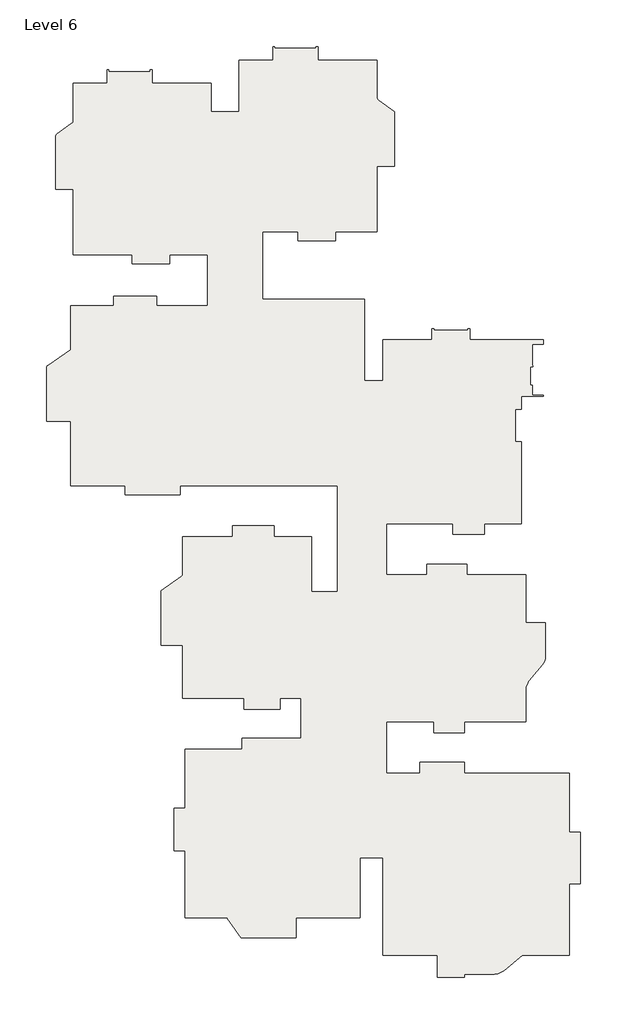
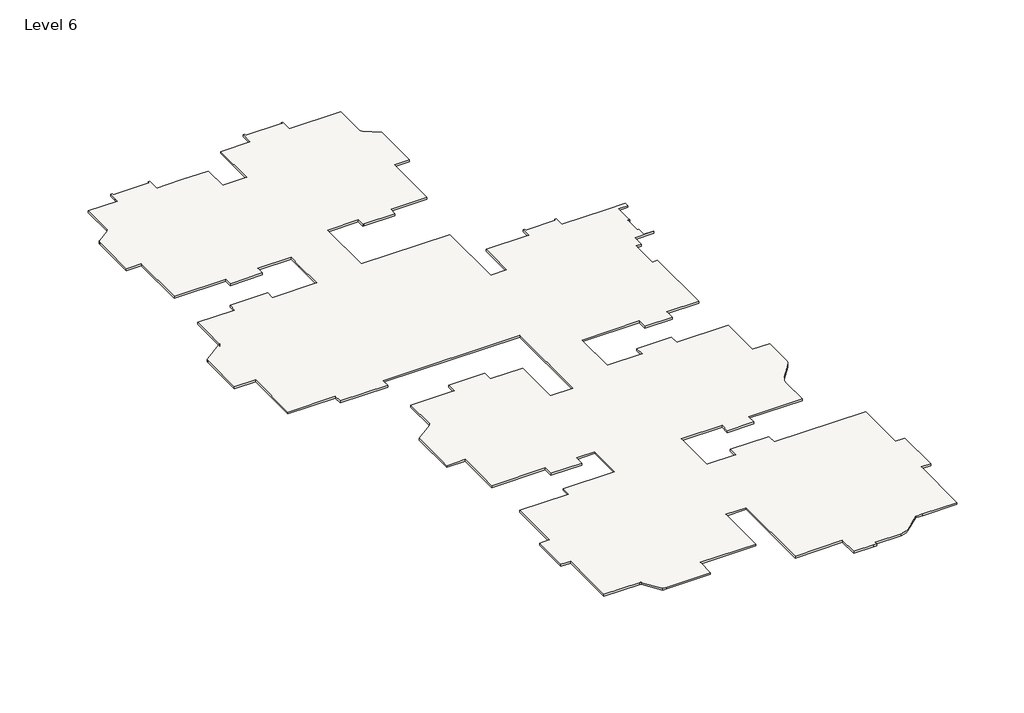
# One storey: 1 slab.
"""IFC4 building model written with IfcOpenShell, lengths in millimetres."""

from ifc_helpers import new_model, si_unit, point, frame, frame_2d, origin, place, context, project, spatial, polyline, circle_curve, trimmed, segment, composite_curve, outline, extrude, element, save

model = new_model("IFC4")

# Units and contexts
model_context = context("Model", 3, world=origin())
ifc_project = project(units=[si_unit("LENGTHUNIT", "METRE", prefix="MILLI")], contexts=[model_context])

# Site, building, storey
site = spatial("IfcSite", under=ifc_project)
building = spatial("IfcBuilding", under=site)
storey = spatial("IfcBuildingStorey", under=building, Name="Level 6", Elevation=9448.8)

# Slab
placement = place(None, origin())
element("IfcSlab", 1, ObjectType="6\" floor", at=placement, inside=storey, context=model_context, shape_type="SweptSolid", body=[
    extrude(outline(composite_curve([segment(polyline([(-9674.5009469, 28521.6416831), (-9674.5009469, 28648.2095876), (-9560.2009469, 28648.2095876), (-9560.2009469, 27756.1461172), (-8800.3399989, 27756.1461172), (-7581.1399989, 27756.1461172), (-5674.0009469, 27756.1461172), (-5674.0009469, 25878.7255084), (-3845.2009469, 25878.7255084), (-3845.2009469, 29269.6255084), (-1617.8862554, 29269.6255084), (-1617.8862554, 30161.6889788), (-1503.5862554, 30161.6889788), (-1503.5862554, 30035.1210743), (1222.0990531, 30035.1210743), (1222.0990531, 30161.6889788), (1336.3990531, 30161.6889788), (1336.3990531, 29269.6255084), (5222.5990531, 29269.6255084), (5222.5990531, 26796.9645799)]), True, "CONTINUOUS"), segment(trimmed(circle_curve(frame_2d((5425.7990531, 26796.9645799)), 203.2), [point((5222.5990531, 26796.9645799))], [point((5309.2715047, 26630.4966536))], True, "CARTESIAN"), True, "CONTINUOUS"), segment(polyline([(5309.2715047, 26630.4966536), (6365.5990531, 25891.0673698), (6365.5990531, 22297.3255084), (5222.5990531, 22297.3255084), (5222.5990531, 18017.4255084), (2479.3990531, 18017.4255084), (2479.3990531, 17431.8689406), (155.2990531, 17431.8689406), (40.9990531, 17431.8689406), (40.9990531, 18017.4255084), (-2288.081873, 18017.4255084), (-2288.081873, 13571.4182723), (4397.0990531, 13571.4182723), (4397.0990531, 8236.2461172), (5616.2990531, 8236.2461172), (5616.2990531, 10928.6450962), (8826.8620119, 10928.6450962), (8826.8620119, 11630.4346228), (8941.1620119, 11630.4346228), (8941.1620119, 11538.2450962), (11198.7752516, 11538.2450962), (11198.7752516, 11630.4346228), (11313.0752516, 11630.4346228), (11313.0752516, 10928.6450962), (14684.0990531, 10928.6450962), (16124.6398221, 10928.6450962), (16124.6398221, 10623.8450962), (15407.9990531, 10623.8450962), (15407.9990531, 9198.1565309), (15440.8254038, 9198.1565309), (15440.8254038, 9147.3565309), (15293.6990531, 9147.3565309), (15293.6990531, 7928.1565309), (15407.9990531, 7928.1565309), (15407.9990531, 7268.4875764), (16124.6398221, 7268.4875764), (16124.6398221, 7211.3375764), (14684.0990531, 7211.3375764), (14684.0990531, 6369.3461172), (14303.0990531, 6369.3461172), (14303.0990531, 5989.8129861), (14303.0990531, 4235.7461172), (14684.0990531, 4235.7461172), (14684.0990531, -1150.3497229), (12281.5704937, -1150.3497229), (12281.5704937, -1861.5497229), (10207.1414203, -1861.5497229), (10207.1414203, -1150.3497229), (5844.8990531, -1150.3497229), (5844.8990531, -4503.1497229), (8478.6664082, -4503.1497229), (8478.6664082, -3803.3538828), (11102.6990531, -3803.3538828), (11102.6990531, -4503.1497229), (14988.8990531, -4503.1497229), (14988.8990531, -7665.4497229), (16284.2990531, -7665.4497229), (16284.2990531, -9831.602777)]), True, "CONTINUOUS"), segment(trimmed(circle_curve(frame_2d((15369.8990531, -9831.602777)), 914.4), [point((16284.2990531, -9831.602777))], [point((16075.314258, -10413.4246987))], False, "CARTESIAN"), True, "CONTINUOUS"), segment(polyline([(16075.314258, -10413.4246987), (15197.8838481, -11477.2429037)]), True, "CONTINUOUS"), segment(trimmed(circle_curve(frame_2d((15903.2990531, -12059.0648255)), 914.4), [point((15197.8838481, -11477.2429037))], [point((14988.8990531, -12059.0648255))], True, "CARTESIAN"), True, "CONTINUOUS"), segment(polyline([(14988.8990531, -12059.0648255), (14988.8990531, -14167.8497229), (10937.0055378, -14167.8497229), (10937.0055378, -14879.0497229), (8943.6990531, -14879.0497229), (8943.6990531, -14167.8497229), (5844.8990531, -14167.8497229), (5844.8990531, -17520.6497229), (8028.4305674, -17520.6497229), (8028.4305674, -16809.4497229), (10950.2990531, -16809.4497229), (10950.2990531, -17520.6497229), (17846.3990531, -17520.6497229), (17846.3990531, -21406.8497229), (18557.5990531, -21406.8497229), (18557.5990531, -24797.7497229), (17846.3990531, -24797.7497229), (17846.3990531, -29484.0497229), (15255.5990531, -29484.0497229), (14750.9761043, -29484.0497229), (13536.5708908, -30485.6833283)]), True, "CONTINUOUS"), segment(trimmed(circle_curve(frame_2d((12809.2934887, -29603.9143222)), 1143.0), [point((13536.5708908, -30485.6833283))], [point((12921.9420983, -30741.3497229))], False, "CARTESIAN"), True, "CONTINUOUS"), segment(polyline([(12921.9420983, -30741.3497229), (10950.2990531, -30741.3497229), (10950.2990531, -30936.1779934), (10721.6990531, -30936.1779934), (9197.6990531, -30936.1779934), (9197.6990531, -29484.0497229), (5616.2990531, -29484.0497229), (5616.2990531, -23083.8583639), (4079.5990531, -23083.8583639), (4079.5990531, -27006.2538828), (-111.4009469, -27006.2538828), (-111.4009469, -28339.7538828), (-3426.1009469, -28339.7538828), (-3705.1428083, -28339.7538828), (-4593.0897712, -27071.2582215)]), True, "CONTINUOUS"), segment(trimmed(circle_curve(frame_2d((-4717.9407159, -27158.6538828)), 152.4), [point((-4593.0897712, -27071.2582215))], [point((-4717.9407159, -27006.2538828))], True, "CARTESIAN"), True, "CONTINUOUS"), segment(polyline([(-4717.9407159, -27006.2538828), (-7388.5009469, -27006.2538828), (-7388.5009469, -22629.8863256), (-8112.4009469, -22629.8863256), (-8112.4009469, -19843.4538828), (-7388.5009469, -19843.4538828), (-7388.5009469, -15957.2538828), (-3654.7009469, -15957.2538828), (-3654.7009469, -15233.3538828), (231.4990531, -15233.3538828), (231.4990531, -12604.4538828), (-1152.8009469, -12604.4538828), (-1152.8009469, -13328.3538828), (-3515.0009469, -13328.3538828), (-3515.0009469, -12604.4538828), (-7553.6009469, -12604.4538828), (-7553.6009469, -9137.3538828), (-8963.3009469, -9137.3538828), (-8963.3009469, -5543.6120214), (-7618.6052856, -4602.3250585)]), True, "CONTINUOUS"), segment(trimmed(circle_curve(frame_2d((-7706.0009469, -4477.4741138)), 152.4), [point((-7618.6052856, -4602.3250585))], [point((-7553.6009469, -4477.4741138))], True, "CARTESIAN"), True, "CONTINUOUS"), segment(polyline([(-7553.6009469, -4477.4741138), (-7553.6009469, -2012.6538828), (-4277.0009469, -2012.6538828), (-4277.0009469, -1288.7538828), (-1533.8009469, -1288.7538828), (-1533.8009469, -2012.6538828), (904.5990531, -2012.6538828), (904.5990531, -5632.1538828), (2631.7990531, -5632.1538828), (2631.7990531, 1340.1461172), (-7726.7333092, 1340.1461172), (-7726.7333092, 730.5461172), (-11312.8009469, 730.5461172), (-11312.8009469, 1340.1461172), (-14894.2009469, 1340.1461172), (-14894.2009469, 5569.2461172), (-16494.4009469, 5569.2461172), (-16494.4009469, 9057.1907685)]), True, "CONTINUOUS"), segment(trimmed(circle_curve(frame_2d((-16291.2009469, 9057.1907685)), 203.2), [point((-16494.4009469, 9057.1907685))], [point((-16407.7284953, 9223.6586947))], False, "CARTESIAN"), True, "CONTINUOUS"), segment(polyline([(-16407.7284953, 9223.6586947), (-14915.8690598, 10267.9602996)]), True, "CONTINUOUS"), segment(trimmed(circle_curve(frame_2d((-14945.0009469, 10309.5772811)), 50.8), [point((-14915.8690598, 10267.9602996))], [point((-14894.2009469, 10309.5772811))], True, "CARTESIAN"), True, "CONTINUOUS"), segment(polyline([(-14894.2009469, 10309.5772811), (-14894.2009469, 13151.1461172), (-12085.9698258, 13151.1461172), (-12085.9698258, 13760.7461172), (-9255.4009469, 13760.7461172), (-9255.4009469, 13151.1461172), (-5902.6009469, 13151.1461172), (-5902.6009469, 15437.1461172), (-5902.6009469, 16503.9461172), (-8417.2009469, 16503.9461172), (-8417.2009469, 15918.3895495), (-10855.6009469, 15918.3895495), (-10855.6009469, 16503.9461172), (-14741.8009469, 16503.9461172), (-14741.8009469, 20783.8461172), (-15884.8009469, 20783.8461172), (-15884.8009469, 24271.7907685)]), True, "CONTINUOUS"), segment(trimmed(circle_curve(frame_2d((-15681.6009469, 24271.7907685)), 203.2), [point((-15884.8009469, 24271.7907685))], [point((-15798.1284953, 24438.2586947))], False, "CARTESIAN"), True, "CONTINUOUS"), segment(polyline([(-15798.1284953, 24438.2586947), (-14828.4733986, 25117.0172625)]), True, "CONTINUOUS"), segment(trimmed(circle_curve(frame_2d((-14945.0009469, 25283.4851887)), 203.2), [point((-14828.4733986, 25117.0172625))], [point((-14741.8009469, 25283.4851887))], True, "CARTESIAN"), True, "CONTINUOUS"), segment(polyline([(-14741.8009469, 25283.4851887), (-14741.8009469, 27756.1461172), (-12514.4862554, 27756.1461172), (-12514.4862554, 28060.9461172), (-12514.4862554, 28648.2095876), (-12400.1862554, 28648.2095876), (-12400.1862554, 28521.6416831), (-9674.5009469, 28521.6416831)]), True, "CONTINUOUS")], self_intersect=False)), frame((0.0, 0.0, 9448.8), z_axis=(0.0, 0.0, 1.0), x_axis=(1.0, 0.0, 0.0)), (0.0, 0.0, 1.0), 152.4),
])

save(model, "model.ifc")

# Revit data of these elements
# Type "6\" floor"
#   Assembly Code = "B1010"
#   Function = 0
#   Layers, outside or top first: 0' - 6" no material (function 1)
# Element 1 (IfcSlab, "6\" floor")
#   Height Offset From Level = 0' - 6"
#   Phase Created = New Construction
#   Materials on its faces: "Default Floor"
# Materials
#   "Default Floor": colour RGB 128 128 128, transparency 0, Cost = 0
